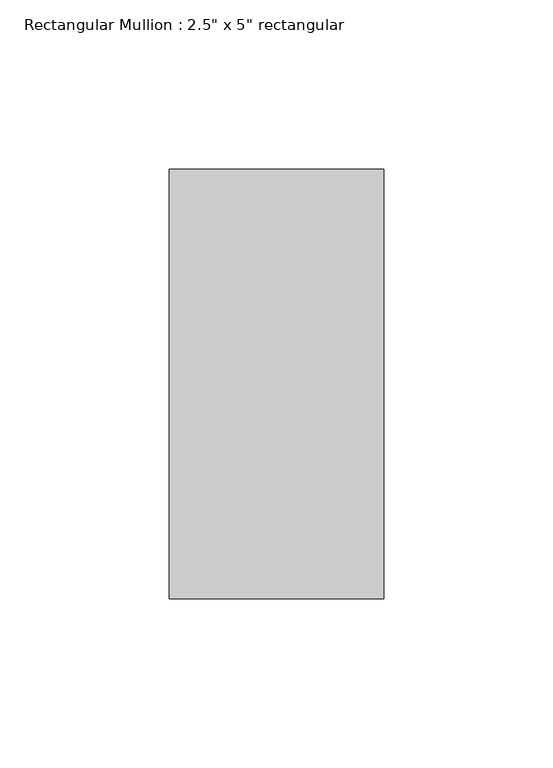
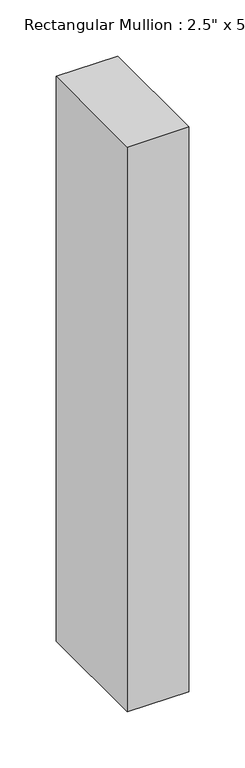
"""IFC4 building model written with IfcOpenShell, lengths in millimetres: member geometry."""

from ifc_helpers import new_model, si_unit, frame, origin, place, context, project, spatial, polyline, outline, extrude, source, transform, mapped, element, save


def member_b73aa13b(model_context):
    return source(origin(), model_context, "Body", "SweptSolid", [
        extrude(outline(polyline([(0.0, 63.5), (0.0, -63.5), (-63.5, -63.5), (-63.5, 63.5), (0.0, 63.5)])), frame((0.0, 0.0, -614.9427475), z_axis=(0.0, 0.0, 1.0), x_axis=(1.0, 0.0, 0.0)), (0.0, 0.0, 1.0), 614.9427475),
    ])


if __name__ == "__main__":
    model = new_model("IFC4")
    model_context = context("Model", 3, world=origin())
    ifc_project = project(units=[si_unit("LENGTHUNIT", "METRE", prefix="MILLI")], contexts=[model_context])
    site = spatial("IfcSite", under=ifc_project)
    building = spatial("IfcBuilding", under=site)
    placement = place(None, origin())
    member_shape = member_b73aa13b(model_context)
    element("IfcMember", 1, ObjectType="Rectangular Mullion : 2.5\" x 5\" rectangular", at=placement, inside=building, context=model_context, shape_type="MappedRepresentation", body=[
        mapped(member_shape, transform((0.0, 0.0, 0.0), x_axis=(1.0, 0.0, 0.0), y_axis=(0.0, 1.0, 0.0), z_axis=(0.0, 0.0, 1.0))),
    ])
    save(model, "model.ifc")

# Revit data of these elements
# Type "Rectangular Mullion : 2.5\" x 5\" rectangular"
#   built-in parameter 1007304 = 0.416667 (stored number, unit not read)
#   built-in parameter 1007301 = 0.104167 (stored number, unit not read)
#   built-in parameter 1007300 = 0.104167 (stored number, unit not read)
# Element 1 (IfcMember, "Rectangular Mullion : 2.5\" x 5\" rectangular")
#   Materials on its faces: "Aluminum"
# Materials
#   "Aluminum": class "Metal", colour RGB 247 247 247, transparency 0, Description = "Aluminum 6061", Cost = 0
